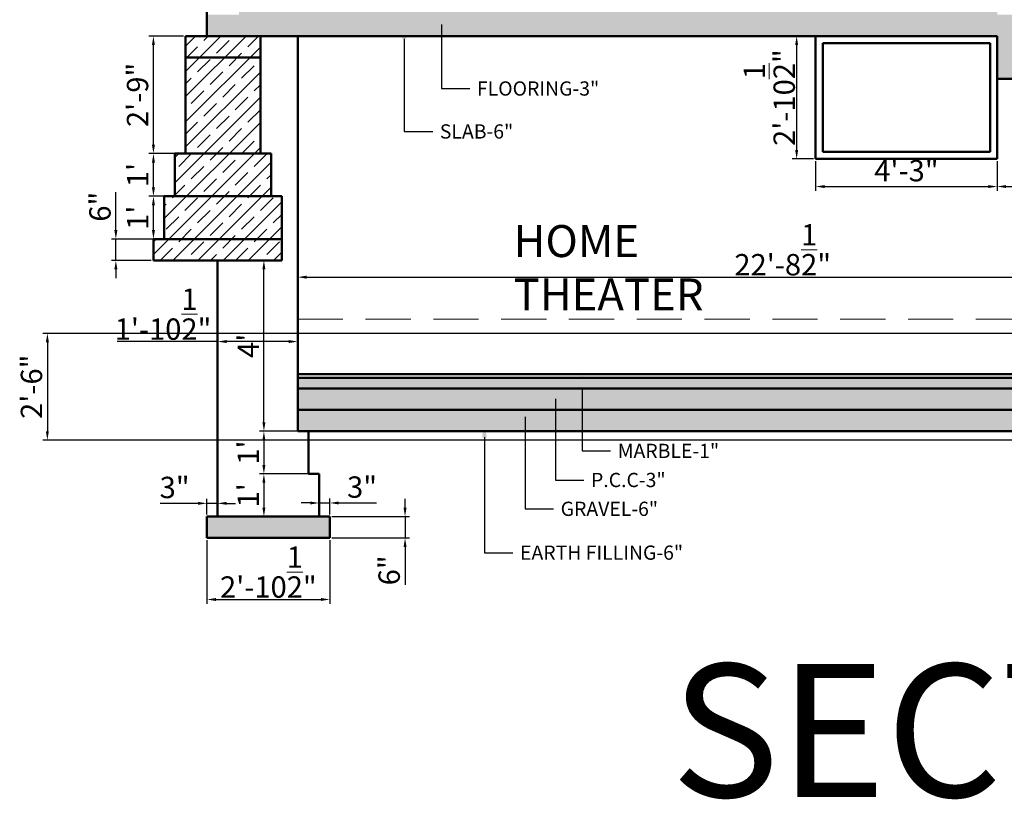
# Model space of a CAD drawing. Units: inches. Extents: x 1615 to 2231, y 1931 to 2519.
# Tile 1 of 6: x 1615 to 1892, y 1931 to 2150. Entities that reach past the tile are written whole.
import ezdxf
from ezdxf import colors
from ezdxf.entities.mleader import LeaderData, LeaderLine
from ezdxf.math import Vec2, Vec3

# ---------------------------------------------------------------- set-up
doc = ezdxf.new("R2010")
doc.units = ezdxf.units.IN
doc.linetypes.add('DASHED', pattern=[19.05, 12.7, -6.35])
for name, color, linetype, lineweight in [('A-ANNO-DIMS', 2, 'Continuous', 18), ('A-ANNO-NOTE', 3, 'Continuous', 18), ('A-ANNO-TEXT', 7, 'Continuous', 35), ('A-AREA-IDEN', 7, 'Continuous', 25), ('A-SECT', 7, 'Continuous', 50), ('A-SECT-HIDN', 8, 'DASHED', 18), ('A-WALL-PATT', 8, 'Continuous', 13), ('C-TOPO-PATT', 252, 'Continuous', 13), ('S-FNDN', 1, 'Continuous', 50), ('S-FNDN-PATT', 8, 'Continuous', 13)]:
    doc.layers.add(name, color=color, linetype=linetype, lineweight=lineweight)
doc.styles.get("Standard").update_dxf_attribs({"font": 'arial.ttf'})
doc.dimstyles.new('ISO-25', dxfattribs={"dimtxt": 6, "dimasz": 2.5, "dimexe": 1.25, "dimexo": 0.625, "dimtad": 1, "dimdec": 1, "dimlunit": 4, "dimtxsty": 'Standard', "dimcen": 2.5, "dimadec": 0, "dimazin": 0, "dimtfac": 1, "dimtdec": 1, "dimtmove": 0, "dimatfit": 3, "dimfxl": 1, "dimarcsym": 0})

# ---------------------------------------------------------------- blocks, each defined once
blk = doc.blocks.new('*D1')
at = {"layer": 'A-ANNO-DIMS', "color": 0, "lineweight": -2, "transparency": 16777216}
for p, q in [((1670.87, 2051.15), (1670.87, 2060.97)), ((1693.37, 2051.15), (1693.37, 2060.97)), ((1670.87, 2059.72), (1642.69, 2059.72)), ((1690.87, 2059.72), (1673.37, 2059.72))]:
    blk.add_line(p, q, dxfattribs=at)
at = {"layer": 'A-ANNO-DIMS', "color": 0, "lineweight": 100, "transparency": 16777216}
for points in [[(1673.37, 2060.14), (1673.37, 2059.31), (1670.87, 2059.72)], [(1690.87, 2060.14), (1690.87, 2059.31), (1693.37, 2059.72)]]:
    blk.add_solid(points, dxfattribs=at)
at = {"layer": 'Defpoints', "color": 0, "lineweight": 100, "transparency": 16777216}
for p in [(1670.87, 2059.72), (1670.87, 2050.53), (1693.37, 2050.53)]:
    blk.add_point(p, dxfattribs=at)
at = {"layer": 'A-ANNO-DIMS', "color": 0, "transparency": 16777216, "insert": (1655.53, 2067.42), "char_height": 6, "attachment_point": 5}
blk.add_mtext('1\'-10{\\H1x;\\S1/2;}"', dxfattribs=at)
blk = doc.blocks.new('*D5')
at = {"layer": 'A-ANNO-DIMS', "color": 0, "lineweight": -2, "transparency": 16777216}
for p, q in [((1642.28, 2091.03), (1642.28, 2101.71)), ((1652.24, 2088.53), (1641.03, 2088.53)), ((1642.28, 2082.53), (1642.28, 2088.53)), ((1652.24, 2082.53), (1641.03, 2082.53)), ((1642.28, 2080.03), (1642.28, 2077.53))]:
    blk.add_line(p, q, dxfattribs=at)
at = {"layer": 'A-ANNO-DIMS', "color": 0, "lineweight": 100, "transparency": 16777216}
for points in [[(1641.86, 2091.03), (1642.7, 2091.03), (1642.28, 2088.53)], [(1641.86, 2080.03), (1642.7, 2080.03), (1642.28, 2082.53)]]:
    blk.add_solid(points, dxfattribs=at)
at = {"layer": 'Defpoints', "color": 0, "lineweight": 100, "transparency": 16777216}
for p in [(1642.28, 2088.53), (1652.87, 2088.53), (1652.87, 2082.53)]:
    blk.add_point(p, dxfattribs=at)
at = {"layer": 'A-ANNO-DIMS', "color": 0, "transparency": 16777216, "insert": (1638.59, 2097.62), "char_height": 6, "attachment_point": 5, "rotation": 90}
blk.add_mtext('6"', dxfattribs=at)
blk = doc.blocks.new('*D6')
at = {"layer": 'A-ANNO-DIMS', "color": 0, "lineweight": -2, "transparency": 16777216}
for p, q in [((1655.24, 2100.53), (1651.58, 2100.53)), ((1652.83, 2091.03), (1652.83, 2098.03)), ((1655.24, 2088.53), (1651.58, 2088.53))]:
    blk.add_line(p, q, dxfattribs=at)
at = {"layer": 'A-ANNO-DIMS', "color": 0, "lineweight": 100, "transparency": 16777216}
for points in [[(1652.42, 2098.03), (1653.25, 2098.03), (1652.83, 2100.53)], [(1652.42, 2091.03), (1653.25, 2091.03), (1652.83, 2088.53)]]:
    blk.add_solid(points, dxfattribs=at)
at = {"layer": 'Defpoints', "color": 0, "lineweight": 100, "transparency": 16777216}
for p in [(1652.83, 2100.53), (1655.87, 2100.53), (1655.87, 2088.53)]:
    blk.add_point(p, dxfattribs=at)
at = {"layer": 'A-ANNO-DIMS', "color": 0, "transparency": 16777216, "insert": (1649.2, 2094.53), "char_height": 6, "attachment_point": 5, "rotation": 90}
blk.add_mtext("1'", dxfattribs=at)
blk = doc.blocks.new('*D7')
at = {"layer": 'A-ANNO-DIMS', "color": 0, "lineweight": -2, "transparency": 16777216}
for p, q in [((1658.24, 2112.53), (1651.58, 2112.53)), ((1652.83, 2103.03), (1652.83, 2110.03)), ((1658.24, 2100.53), (1651.58, 2100.53))]:
    blk.add_line(p, q, dxfattribs=at)
at = {"layer": 'A-ANNO-DIMS', "color": 0, "lineweight": 100, "transparency": 16777216}
for points in [[(1652.42, 2110.03), (1653.25, 2110.03), (1652.83, 2112.53)], [(1652.42, 2103.03), (1653.25, 2103.03), (1652.83, 2100.53)]]:
    blk.add_solid(points, dxfattribs=at)
at = {"layer": 'Defpoints', "color": 0, "lineweight": 100, "transparency": 16777216}
for p in [(1652.83, 2112.53), (1658.87, 2112.53), (1658.87, 2100.53)]:
    blk.add_point(p, dxfattribs=at)
at = {"layer": 'A-ANNO-DIMS', "color": 0, "transparency": 16777216, "insert": (1649.2, 2106.53), "char_height": 6, "attachment_point": 5, "rotation": 90}
blk.add_mtext("1'", dxfattribs=at)
blk = doc.blocks.new('*D8')
at = {"layer": 'A-ANNO-DIMS', "color": 0, "lineweight": -2, "transparency": 16777216}
for p, q in [((1661.24, 2145.53), (1651.58, 2145.53)), ((1652.83, 2115.03), (1652.83, 2143.03)), ((1661.24, 2112.53), (1651.58, 2112.53))]:
    blk.add_line(p, q, dxfattribs=at)
at = {"layer": 'A-ANNO-DIMS', "color": 0, "lineweight": 100, "transparency": 16777216}
for points in [[(1652.42, 2143.03), (1653.25, 2143.03), (1652.83, 2145.53)], [(1652.42, 2115.03), (1653.25, 2115.03), (1652.83, 2112.53)]]:
    blk.add_solid(points, dxfattribs=at)
at = {"layer": 'Defpoints', "color": 0, "lineweight": 100, "transparency": 16777216}
for p in [(1652.83, 2145.53), (1661.87, 2145.53), (1661.87, 2112.53)]:
    blk.add_point(p, dxfattribs=at)
at = {"layer": 'A-ANNO-DIMS', "color": 0, "transparency": 16777216, "insert": (1649.15, 2129.03), "char_height": 6, "attachment_point": 5, "rotation": 90}
blk.add_mtext('2\'-9"', dxfattribs=at)
blk = doc.blocks.new('*D9')
at = {"layer": 'A-ANNO-DIMS', "color": 0, "lineweight": -2, "transparency": 16777216}
for p, q in [((1693.37, 2070.69), (1693.37, 2079.07)), ((1695.87, 2077.82), (1963.37, 2077.82)), ((1965.87, 2070.69), (1965.87, 2079.07))]:
    blk.add_line(p, q, dxfattribs=at)
at = {"layer": 'A-ANNO-DIMS', "color": 0, "lineweight": 100, "transparency": 16777216}
for points in [[(1695.87, 2078.24), (1695.87, 2077.4), (1693.37, 2077.82)], [(1963.37, 2078.24), (1963.37, 2077.4), (1965.87, 2077.82)]]:
    blk.add_solid(points, dxfattribs=at)
at = {"layer": 'Defpoints', "color": 0, "lineweight": 100, "transparency": 16777216}
for p in [(1965.87, 2077.82), (1693.37, 2070.06), (1965.87, 2070.06)]:
    blk.add_point(p, dxfattribs=at)
at = {"layer": 'A-ANNO-DIMS', "color": 0, "transparency": 16777216, "insert": (1829.62, 2085.52), "char_height": 6, "attachment_point": 5}
blk.add_mtext('22\'-8{\\H1x;\\S1/2;}"', dxfattribs=at)
blk = doc.blocks.new('*D11')
at = {"layer": 'A-ANNO-DIMS', "color": 0, "lineweight": -2, "transparency": 16777216}
for p, q in [((1688.24, 2082.53), (1682.62, 2082.53)), ((1683.87, 2037.03), (1683.87, 2080.03)), ((1692.74, 2034.53), (1682.62, 2034.53))]:
    blk.add_line(p, q, dxfattribs=at)
at = {"layer": 'A-ANNO-DIMS', "color": 0, "lineweight": 100, "transparency": 16777216}
for points in [[(1683.45, 2080.03), (1684.28, 2080.03), (1683.87, 2082.53)], [(1683.45, 2037.03), (1684.28, 2037.03), (1683.87, 2034.53)]]:
    blk.add_solid(points, dxfattribs=at)
at = {"layer": 'Defpoints', "color": 0, "lineweight": 100, "transparency": 16777216}
for p in [(1683.87, 2082.53), (1688.87, 2082.53), (1693.37, 2034.53)]:
    blk.add_point(p, dxfattribs=at)
at = {"layer": 'A-ANNO-DIMS', "color": 0, "transparency": 16777216, "insert": (1680.24, 2058.53), "char_height": 6, "attachment_point": 5, "rotation": 90}
blk.add_mtext("4'", dxfattribs=at)
blk = doc.blocks.new('*D12')
at = {"layer": 'A-ANNO-DIMS', "color": 0, "lineweight": -2, "transparency": 16777216}
for p, q in [((1695.74, 2034.53), (1682.62, 2034.53)), ((1683.87, 2032.03), (1683.87, 2025.03)), ((1695.74, 2022.53), (1682.62, 2022.53))]:
    blk.add_line(p, q, dxfattribs=at)
at = {"layer": 'A-ANNO-DIMS', "color": 0, "lineweight": 100, "transparency": 16777216}
for points in [[(1683.45, 2032.03), (1684.28, 2032.03), (1683.87, 2034.53)], [(1683.45, 2025.03), (1684.28, 2025.03), (1683.87, 2022.53)]]:
    blk.add_solid(points, dxfattribs=at)
at = {"layer": 'Defpoints', "color": 0, "lineweight": 100, "transparency": 16777216}
for p in [(1696.37, 2034.53), (1683.87, 2022.53), (1696.37, 2022.53)]:
    blk.add_point(p, dxfattribs=at)
at = {"layer": 'A-ANNO-DIMS', "color": 0, "transparency": 16777216, "insert": (1680.23, 2028.53), "char_height": 6, "attachment_point": 5, "rotation": 90}
blk.add_mtext("1'", dxfattribs=at)
blk = doc.blocks.new('*D13')
at = {"layer": 'A-ANNO-DIMS', "color": 0, "lineweight": -2, "transparency": 16777216}
for p, q in [((1698.74, 2022.53), (1682.62, 2022.53)), ((1683.87, 2020.03), (1683.87, 2013.03)), ((1698.74, 2010.53), (1682.62, 2010.53))]:
    blk.add_line(p, q, dxfattribs=at)
at = {"layer": 'A-ANNO-DIMS', "color": 0, "lineweight": 100, "transparency": 16777216}
for points in [[(1683.45, 2020.03), (1684.28, 2020.03), (1683.87, 2022.53)], [(1683.45, 2013.03), (1684.28, 2013.03), (1683.87, 2010.53)]]:
    blk.add_solid(points, dxfattribs=at)
at = {"layer": 'Defpoints', "color": 0, "lineweight": 100, "transparency": 16777216}
for p in [(1699.37, 2022.53), (1683.87, 2010.53), (1699.37, 2010.53)]:
    blk.add_point(p, dxfattribs=at)
at = {"layer": 'A-ANNO-DIMS', "color": 0, "transparency": 16777216, "insert": (1680.23, 2016.53), "char_height": 6, "attachment_point": 5, "rotation": 90}
blk.add_mtext("1'", dxfattribs=at)
blk = doc.blocks.new('*D14')
at = {"layer": 'A-ANNO-DIMS', "color": 0, "lineweight": -2, "transparency": 16777216}
for p, q in [((1667.87, 2003.9), (1667.87, 1986)), ((1702.37, 2003.9), (1702.37, 1986)), ((1670.37, 1987.25), (1699.87, 1987.25))]:
    blk.add_line(p, q, dxfattribs=at)
at = {"layer": 'A-ANNO-DIMS', "color": 0, "lineweight": 100, "transparency": 16777216}
for points in [[(1670.37, 1987.67), (1670.37, 1986.84), (1667.87, 1987.25)], [(1699.87, 1987.67), (1699.87, 1986.84), (1702.37, 1987.25)]]:
    blk.add_solid(points, dxfattribs=at)
at = {"layer": 'Defpoints', "color": 0, "lineweight": 100, "transparency": 16777216}
for p in [(1667.87, 2004.53), (1702.37, 2004.53), (1702.37, 1987.25)]:
    blk.add_point(p, dxfattribs=at)
at = {"layer": 'A-ANNO-DIMS', "color": 0, "transparency": 16777216, "insert": (1685.12, 1994.95), "char_height": 6, "attachment_point": 5}
blk.add_mtext('2\'-10{\\H1x;\\S1/2;}"', dxfattribs=at)
blk = doc.blocks.new('*D15')
at = {"layer": 'A-ANNO-DIMS', "color": 0, "lineweight": -2, "transparency": 16777216}
for p, q in [((1696.87, 2014.37), (1694.37, 2014.37)), ((1699.37, 2011.15), (1699.37, 2015.62)), ((1699.37, 2014.37), (1702.37, 2014.37)), ((1702.37, 2011.15), (1702.37, 2015.62)), ((1704.87, 2014.37), (1715.51, 2014.37))]:
    blk.add_line(p, q, dxfattribs=at)
at = {"layer": 'A-ANNO-DIMS', "color": 0, "lineweight": 100, "transparency": 16777216}
for points in [[(1696.87, 2014.78), (1696.87, 2013.95), (1699.37, 2014.37)], [(1704.87, 2014.78), (1704.87, 2013.95), (1702.37, 2014.37)]]:
    blk.add_solid(points, dxfattribs=at)
at = {"layer": 'Defpoints', "color": 0, "lineweight": 100, "transparency": 16777216}
for p in [(1702.37, 2014.37), (1699.37, 2010.53), (1702.37, 2010.53)]:
    blk.add_point(p, dxfattribs=at)
at = {"layer": 'A-ANNO-DIMS', "color": 0, "transparency": 16777216, "insert": (1711.44, 2018.06), "char_height": 6, "attachment_point": 5}
blk.add_mtext('3"', dxfattribs=at)
blk = doc.blocks.new('*D16')
at = {"layer": 'A-ANNO-DIMS', "color": 0, "lineweight": -2, "transparency": 16777216}
for p, q in [((1665.37, 2014.26), (1654.72, 2014.26)), ((1667.87, 2011.15), (1667.87, 2015.51)), ((1670.87, 2014.26), (1667.87, 2014.26)), ((1670.87, 2011.15), (1670.87, 2015.51)), ((1673.37, 2014.26), (1675.87, 2014.26))]:
    blk.add_line(p, q, dxfattribs=at)
at = {"layer": 'A-ANNO-DIMS', "color": 0, "lineweight": 100, "transparency": 16777216}
for points in [[(1665.37, 2014.68), (1665.37, 2013.85), (1667.87, 2014.26)], [(1673.37, 2014.68), (1673.37, 2013.85), (1670.87, 2014.26)]]:
    blk.add_solid(points, dxfattribs=at)
at = {"layer": 'Defpoints', "color": 0, "lineweight": 100, "transparency": 16777216}
for p in [(1667.87, 2014.26), (1667.87, 2010.53), (1670.87, 2010.53)]:
    blk.add_point(p, dxfattribs=at)
at = {"layer": 'A-ANNO-DIMS', "color": 0, "transparency": 16777216, "insert": (1658.79, 2017.95), "char_height": 6, "attachment_point": 5}
blk.add_mtext('3"', dxfattribs=at)
blk = doc.blocks.new('*D23')
at = {"layer": 'A-ANNO-DIMS', "color": 0, "lineweight": -2, "transparency": 16777216}
for p, q in [((1838.24, 2145.53), (1832.28, 2145.53)), ((1833.53, 2143.03), (1833.53, 2113.53)), ((1838.24, 2111.03), (1832.28, 2111.03))]:
    blk.add_line(p, q, dxfattribs=at)
at = {"layer": 'A-ANNO-DIMS', "color": 0, "lineweight": 100, "transparency": 16777216}
for points in [[(1833.11, 2143.03), (1833.95, 2143.03), (1833.53, 2145.53)], [(1833.11, 2113.53), (1833.95, 2113.53), (1833.53, 2111.03)]]:
    blk.add_solid(points, dxfattribs=at)
at = {"layer": 'Defpoints', "color": 0, "lineweight": 100, "transparency": 16777216}
for p in [(1838.87, 2145.53), (1833.53, 2111.03), (1838.87, 2111.03)]:
    blk.add_point(p, dxfattribs=at)
at = {"layer": 'A-ANNO-DIMS', "color": 0, "transparency": 16777216, "insert": (1825.83, 2128.28), "char_height": 6, "attachment_point": 5, "rotation": 90}
blk.add_mtext('2\'-10{\\H1x;\\S1/2;}"', dxfattribs=at)
blk = doc.blocks.new('*D24')
at = {"layer": 'A-ANNO-DIMS', "color": 0, "lineweight": -2, "transparency": 16777216}
for p, q in [((1838.87, 2110.4), (1838.87, 2102.03)), ((1889.87, 2110.4), (1889.87, 2102.03)), ((1841.37, 2103.28), (1887.37, 2103.28))]:
    blk.add_line(p, q, dxfattribs=at)
at = {"layer": 'A-ANNO-DIMS', "color": 0, "lineweight": 100, "transparency": 16777216}
for points in [[(1841.37, 2103.7), (1841.37, 2102.86), (1838.87, 2103.28)], [(1887.37, 2103.7), (1887.37, 2102.86), (1889.87, 2103.28)]]:
    blk.add_solid(points, dxfattribs=at)
at = {"layer": 'Defpoints', "color": 0, "lineweight": 100, "transparency": 16777216}
for p in [(1838.87, 2111.03), (1889.87, 2111.03), (1889.87, 2103.28)]:
    blk.add_point(p, dxfattribs=at)
at = {"layer": 'A-ANNO-DIMS', "color": 0, "transparency": 16777216, "insert": (1864.37, 2106.97), "char_height": 6, "attachment_point": 5}
blk.add_mtext('4\'-3"', dxfattribs=at)
blk = doc.blocks.new('*D26')
at = {"layer": 'A-ANNO-DIMS', "color": 0, "lineweight": -2, "transparency": 16777216}
for p, q in [((1889.87, 2110.4), (1889.87, 2102.03)), ((1965.87, 2110.4), (1965.87, 2102.03)), ((1892.37, 2103.28), (1963.37, 2103.28))]:
    blk.add_line(p, q, dxfattribs=at)
at = {"layer": 'A-ANNO-DIMS', "color": 0, "lineweight": 100, "transparency": 16777216}
for points in [[(1892.37, 2103.7), (1892.37, 2102.86), (1889.87, 2103.28)], [(1963.37, 2103.7), (1963.37, 2102.86), (1965.87, 2103.28)]]:
    blk.add_solid(points, dxfattribs=at)
at = {"layer": 'Defpoints', "color": 0, "lineweight": 100, "transparency": 16777216}
for p in [(1889.87, 2111.03), (1965.87, 2111.03), (1965.87, 2103.28)]:
    blk.add_point(p, dxfattribs=at)
at = {"layer": 'A-ANNO-DIMS', "color": 0, "transparency": 16777216, "insert": (1927.87, 2106.97), "char_height": 6, "attachment_point": 5}
blk.add_mtext('6\'-4"', dxfattribs=at)
blk = doc.blocks.new('*D74')
at = {"layer": 'A-ANNO-DIMS', "color": 0, "lineweight": -2, "transparency": 16777216}
for p, q in [((1723.52, 2013.03), (1723.52, 2015.53)), ((1702.99, 2010.53), (1724.77, 2010.53)), ((1723.52, 2010.53), (1723.52, 2004.53)), ((1702.99, 2004.53), (1724.77, 2004.53)), ((1723.52, 2002.03), (1723.52, 1991.35))]:
    blk.add_line(p, q, dxfattribs=at)
at = {"layer": 'A-ANNO-DIMS', "color": 0, "lineweight": 100, "transparency": 16777216}
for points in [[(1723.1, 2013.03), (1723.94, 2013.03), (1723.52, 2010.53)], [(1723.1, 2002.03), (1723.94, 2002.03), (1723.52, 2004.53)]]:
    blk.add_solid(points, dxfattribs=at)
at = {"layer": 'Defpoints', "color": 0, "lineweight": 100, "transparency": 16777216}
for p in [(1702.37, 2010.53), (1702.37, 2004.53), (1723.52, 2004.53)]:
    blk.add_point(p, dxfattribs=at)
at = {"layer": 'A-ANNO-DIMS', "color": 0, "transparency": 16777216, "insert": (1719.83, 1995.44), "char_height": 6, "attachment_point": 5, "rotation": 90}
blk.add_mtext('6"', dxfattribs=at)
blk = doc.blocks.new('*D88')
at = {"layer": 'A-ANNO-DIMS', "color": 0, "lineweight": -2, "transparency": 16777216}
for p, q in [((2162.74, 2062.03), (1621.79, 2062.03)), ((1623.04, 2059.53), (1623.04, 2034.53)), ((2165.74, 2032.03), (1621.79, 2032.03))]:
    blk.add_line(p, q, dxfattribs=at)
at = {"layer": 'A-ANNO-DIMS', "color": 0, "lineweight": 100, "transparency": 16777216}
for points in [[(1622.62, 2059.53), (1623.46, 2059.53), (1623.04, 2062.03)], [(1622.62, 2034.53), (1623.46, 2034.53), (1623.04, 2032.03)]]:
    blk.add_solid(points, dxfattribs=at)
at = {"layer": 'Defpoints', "color": 0, "lineweight": 100, "transparency": 16777216}
for p in [(2163.37, 2062.03), (1623.04, 2032.03), (2166.37, 2032.03)]:
    blk.add_point(p, dxfattribs=at)
at = {"layer": 'A-ANNO-DIMS', "color": 0, "transparency": 16777216, "insert": (1619.35, 2047.03), "char_height": 6, "attachment_point": 5, "rotation": 90}
blk.add_mtext('2\'-6"', dxfattribs=at)

msp = doc.modelspace()

# ---------------------------------------------------------------- hatches: boundary and pattern name
at = {"layer": 'A-WALL-PATT'}
h = msp.add_hatch(dxfattribs=at)
h.set_pattern_fill('DOTS', color=256, scale=0.5)
h.paths.add_polyline_path([(2142.37, 2442.53), (1839.37, 2442.53), (1676.87, 2442.53), (1676.87, 2439.53), (2142.37, 2439.53)])
h.paths.add_polyline_path([(1889.87, 2298.53), (1676.87, 2298.53), (1676.87, 2295.53), (1889.87, 2295.53)])
h.paths.add_polyline_path([(2142.37, 2298.53), (1974.87, 2298.53), (1974.87, 2295.53), (2142.37, 2295.53)])
h.paths.add_polyline_path([(1889.87, 2154.53), (1676.87, 2154.53), (1676.87, 2151.53), (1889.87, 2151.53)])
h.paths.add_polyline_path([(1965.87, 2154.53), (1894.37, 2154.53), (1894.37, 2151.53), (1965.87, 2151.53)])
h.paths.add_polyline_path([(2142.37, 2154.53), (1974.87, 2154.53), (1974.87, 2151.53), (2142.37, 2151.53)])
h.paths.add_polyline_path([(2094.37, 2062.03), (1974.87, 2062.03), (1974.87, 2059.03), (2094.37, 2059.03)])
h.paths.add_polyline_path([(2142.37, 2062.03), (2098.87, 2062.03), (2098.87, 2059.03), (2142.37, 2059.03)])
h.paths.add_polyline_path([(1956.87, 2049.53), (1693.37, 2049.53), (1693.37, 2046.53), (1956.87, 2046.53)])
h = msp.add_hatch(dxfattribs=at)
h.set_pattern_fill('AR-CONC', color=256, scale=0.1)
h.paths.add_polyline_path([(1898.87, 2151.53), (1667.87, 2151.53), (1667.87, 2145.53), (1679.87, 2145.53), (1682.87, 2145.53), (1889.87, 2145.53), (1889.87, 2133.53), (1974.87, 2133.53), (1974.87, 2145.53), (2142.37, 2145.53), (2142.37, 2133.53), (2157.37, 2133.53), (2157.37, 2151.53), (2155.87, 2151.53), (2151.37, 2151.53), (1965.87, 2151.53), (1965.87, 2139.53), (1898.87, 2139.53)])
h.paths.add_polyline_path([(1898.87, 2295.53), (1667.87, 2295.53), (1667.87, 2277.53), (1676.87, 2277.53), (1676.87, 2289.53), (1889.87, 2289.53), (1889.87, 2277.53), (1974.87, 2277.53), (1974.87, 2289.53), (2142.37, 2289.53), (2142.37, 2277.53), (2151.37, 2277.53), (2151.37, 2295.53), (1965.87, 2295.53), (1965.87, 2283.53), (1898.87, 2283.53)])
h.paths.add_polyline_path([(2142.37, 2439.53), (1676.87, 2439.53), (1667.87, 2439.53), (1667.87, 2421.53), (1676.87, 2421.53), (1676.87, 2433.53), (1889.87, 2433.53), (1889.87, 2421.29), (1898.87, 2421.29), (1898.87, 2433.53), (1965.87, 2433.53), (1965.87, 2421.29), (1974.87, 2421.29), (1974.87, 2433.53), (2142.37, 2433.53)])
h = msp.add_hatch(dxfattribs=at)
h.set_pattern_fill('JIS_STN_1E', color=256, scale=5)
h.paths.add_polyline_path([(1688.87, 2100.53), (1655.87, 2100.53), (1655.87, 2088.53), (1688.87, 2088.53)])
h.paths.add_polyline_path([(1685.87, 2112.53), (1658.87, 2112.53), (1658.87, 2100.53), (1685.87, 2100.53)])
h.paths.add_polyline_path([(1682.87, 2139.53), (1661.87, 2139.53), (1661.87, 2112.53), (1682.87, 2112.53)])
h.paths.add_polyline_path([(1688.87, 2088.53), (1655.87, 2088.53), (1652.87, 2088.53), (1652.87, 2082.53), (1688.87, 2082.53)])
h.paths.add_polyline_path([(1682.87, 2145.53), (1679.87, 2145.53), (1676.87, 2145.53), (1661.87, 2145.53), (1661.87, 2139.53), (1682.87, 2139.53)])
h.paths.add_polyline_path([(1974.87, 2057.03), (1956.87, 2057.03), (1956.87, 2044.03), (1974.87, 2044.03)])
h.paths.add_polyline_path([(1974.87, 2060.03), (1956.87, 2060.03), (1956.87, 2057.03), (1974.87, 2057.03)])
h.paths.add_polyline_path([(1980.87, 2032.03), (1950.87, 2032.03), (1950.87, 2020.03), (1980.87, 2020.03)])
h.paths.add_polyline_path([(1977.87, 2044.03), (1953.87, 2044.03), (1953.87, 2032.03), (1977.87, 2032.03)])
h.paths.add_polyline_path([(1983.87, 2020.03), (1947.87, 2020.03), (1947.87, 2008.03), (1983.87, 2008.03)])
h.paths.add_polyline_path([(2104.12, 2056.03), (2089.12, 2056.03), (2089.12, 2032.03), (2104.12, 2032.03)])
h.paths.add_polyline_path([(2104.12, 2059.03), (2089.12, 2059.03), (2089.12, 2056.03), (2104.12, 2056.03)])
h.paths.add_polyline_path([(2105.62, 2032.03), (2087.62, 2032.03), (2087.62, 2020.03), (2105.62, 2020.03)])
h.paths.add_polyline_path([(2107.12, 2020.03), (2086.12, 2020.03), (2086.12, 2008.03), (2107.12, 2008.03)])
h.paths.add_polyline_path([(2169.37, 2032.03), (2139.37, 2032.03), (2139.37, 2020.03), (2169.37, 2020.03)])
h.paths.add_polyline_path([(2172.37, 2020.03), (2136.37, 2020.03), (2136.37, 2008.03), (2172.37, 2008.03)])
h.paths.add_polyline_path([(2166.37, 2062.03), (2163.37, 2062.03), (2163.37, 2089.03), (2160.37, 2089.03), (2160.37, 2112.53), (2157.37, 2112.53), (2157.37, 2133.53), (2142.37, 2133.53), (2142.37, 2032.03), (2166.37, 2032.03)])
at = {"layer": 'C-TOPO-PATT'}
h = msp.add_hatch(dxfattribs=at)
h.set_pattern_fill('GRAVEL', color=256, scale=0.5, angle=27)
h.paths.add_polyline_path([(1956.87, 2046.53), (1693.37, 2046.53), (1693.37, 2040.53), (1953.87, 2040.53), (1953.87, 2044.03), (1956.87, 2044.03)])
h.paths.add_polyline_path([(2089.12, 2059.03), (1974.87, 2059.03), (1974.87, 2053.03), (2089.12, 2053.03)])
h.paths.add_polyline_path([(2142.37, 2059.03), (2104.12, 2059.03), (2104.12, 2053.03), (2142.37, 2053.03)])
h.paths.add_polyline_path([(2195.62, 2124.53), (2157.37, 2124.53), (2157.37, 2118.53), (2195.62, 2118.53)])
h = msp.add_hatch(dxfattribs=at)
h.set_pattern_fill('EARTH', color=256, angle=27)
h.paths.add_polyline_path([(1953.87, 2040.53), (1693.37, 2040.53), (1693.37, 2034.53), (1696.37, 2034.53), (1953.87, 2034.53)])
h.paths.add_polyline_path([(2089.12, 2053.03), (1974.87, 2053.03), (1974.87, 2047.03), (2089.12, 2047.03)])
h.paths.add_polyline_path([(2142.37, 2053.03), (2104.12, 2053.03), (2104.12, 2047.03), (2142.37, 2047.03)])
at = {"layer": 'S-FNDN-PATT'}
h = msp.add_hatch(dxfattribs=at)
h.set_pattern_fill('AR-CONC', color=256, scale=0.1)
h.paths.add_polyline_path([(1702.37, 2010.53), (1667.87, 2010.53), (1667.87, 2004.53), (1702.37, 2004.53)])
h.paths.add_polyline_path([(1986.87, 2008.03), (1944.87, 2008.03), (1944.87, 2002.03), (1986.87, 2002.03)])
h.paths.add_polyline_path([(2108.62, 2008.03), (2084.62, 2008.03), (2084.62, 2002.03), (2108.62, 2002.03)])
h.paths.add_polyline_path([(2175.37, 2008.03), (2133.37, 2008.03), (2133.37, 2002.03), (2175.37, 2002.03)])

# ---------------------------------------------------------------- linework, layer by layer
at = {"layer": 'A-SECT'}
for p, q in [((1667.87, 2476.53), (1667.87, 2145.53)), ((1679.87, 2145.53), (1661.87, 2145.53)), ((1661.87, 2145.53), (1661.87, 2112.53)), ((1667.87, 2145.53), (1676.87, 2145.53)), ((1676.87, 2145.53), (1889.87, 2145.53)), ((1682.87, 2145.53), (1679.87, 2145.53)), ((1682.87, 2139.53), (1682.87, 2145.53)), ((1693.37, 2145.53), (1693.37, 2034.53)), ((1838.87, 2145.53), (1838.87, 2111.03)), ((1889.87, 2145.53), (1889.87, 2133.53)), ((1840.87, 2143.53), (1887.87, 2143.53)), ((1840.87, 2143.53), (1840.87, 2113.03)), ((1887.87, 2143.53), (1887.87, 2133.53)), ((1682.87, 2139.53), (1661.87, 2139.53)), ((1682.87, 2139.53), (1682.87, 2112.53)), ((1887.87, 2113.03), (1887.87, 2133.53)), ((1889.87, 2133.53), (1974.87, 2133.53)), ((1889.87, 2111.03), (1889.87, 2133.53)), ((1838.87, 2111.03), (1889.87, 2111.03)), ((1840.87, 2113.03), (1887.87, 2113.03)), ((1693.37, 2050.53), (1956.87, 2050.53)), ((1693.37, 2049.53), (1956.87, 2049.53)), ((1693.37, 2046.53), (1956.87, 2046.53)), ((1693.37, 2040.53), (1953.87, 2040.53))]:
    msp.add_line(p, q, dxfattribs=at)
at = {"layer": 'A-SECT-HIDN'}
msp.add_line((1693.37, 2066.03), (1965.87, 2066.03), dxfattribs=at)
at = {"layer": 'S-FNDN'}
for p, q in [((1685.87, 2112.53), (1658.87, 2112.53)), ((1658.87, 2112.53), (1658.87, 2100.53)), ((1685.87, 2112.53), (1685.87, 2100.53)), ((1688.87, 2100.53), (1655.87, 2100.53)), ((1655.87, 2100.53), (1655.87, 2088.53)), ((1688.87, 2100.53), (1688.87, 2088.53)), ((1688.87, 2088.53), (1652.87, 2088.53)), ((1652.87, 2088.53), (1652.87, 2082.53)), ((1688.87, 2082.53), (1688.87, 2088.53)), ((1652.87, 2082.53), (1688.87, 2082.53)), ((1670.87, 2082.53), (1670.87, 2010.53)), ((1696.37, 2034.53), (1693.37, 2034.53)), ((1696.37, 2034.53), (1696.37, 2022.53)), ((1696.37, 2034.53), (1953.87, 2034.53)), ((1699.37, 2022.53), (1696.37, 2022.53)), ((1699.37, 2022.53), (1699.37, 2010.53)), ((1702.37, 2010.53), (1667.87, 2010.53)), ((1667.87, 2010.53), (1667.87, 2004.53)), ((1702.37, 2004.53), (1702.37, 2010.53)), ((1667.87, 2004.53), (1702.37, 2004.53))]:
    msp.add_line(p, q, dxfattribs=at)

# ---------------------------------------------------------------- texts
at = {"layer": 'A-ANNO-TEXT'}
msp.add_text('SECTION', height=37.358, dxfattribs=at).set_placement((1798.24, 1931.77))
at = {"layer": 'A-AREA-IDEN', "insert": (1754.02, 2092.46), "char_height": 9, "attachment_point": 1}
msp.add_mtext_dynamic_manual_height_columns('HOME THEATER', width=38.6979, gutter_width=12.5, heights=[0], dxfattribs=at)

# ---------------------------------------------------------------- dimensions: what is measured, and where the dimension line sits
at = {"layer": 'A-ANNO-DIMS'}
for base, p1, p2, override, picture, middle in [((1652.83, 2145.53), (1661.87, 2112.53), (1661.87, 2145.53), {"dimclrd": 0, "dimclre": 0, "dimclrt": 0}, '*D8', (1649.15, 2129.03)), ((1833.53, 2111.03), (1838.87, 2145.53), (1838.87, 2111.03), {"dimclrd": 0, "dimclre": 0, "dimclrt": 0}, '*D23', (1825.83, 2128.28)), ((1652.83, 2112.53), (1658.87, 2100.53), (1658.87, 2112.53), {"dimclrd": 0, "dimclre": 0, "dimclrt": 0}, '*D7', (1649.2, 2106.53)), ((1642.28, 2088.53), (1652.87, 2082.53), (1652.87, 2088.53), {"dimclrd": 0, "dimclre": 0, "dimclrt": 0}, '*D5', (1638.59, 2097.62)), ((1652.83, 2100.53), (1655.87, 2088.53), (1655.87, 2100.53), {"dimclrd": 0, "dimclre": 0, "dimclrt": 0}, '*D6', (1649.2, 2094.53)), ((1683.87, 2082.53), (1693.37, 2034.53), (1688.87, 2082.53), {"dimclrd": 0, "dimclre": 0, "dimclrt": 0}, '*D11', (1680.24, 2058.53)), ((1623.04, 2032.03), (2163.37, 2062.03), (2166.37, 2032.03), {"dimdec": 1, "dimlfac": 1, "dimrnd": 0, "dimzin": 1, "dimdsep": 46, "dimlunit": 4, "dimfrac": 2}, '*D88', (1619.35, 2047.03)), ((1683.87, 2022.53), (1696.37, 2034.53), (1696.37, 2022.53), {"dimclrd": 0, "dimclre": 0, "dimclrt": 0}, '*D12', (1680.23, 2028.53)), ((1683.87, 2010.53), (1699.37, 2022.53), (1699.37, 2010.53), {"dimclrd": 0, "dimclre": 0, "dimclrt": 0}, '*D13', (1680.23, 2016.53)), ((1723.52, 2004.53), (1702.37, 2010.53), (1702.37, 2004.53), {"dimclrd": 0, "dimclre": 0, "dimclrt": 0}, '*D74', (1719.83, 1995.44))]:
    dim = msp.add_linear_dim(base=base, p1=p1, p2=p2, angle=90, dimstyle='ISO-25', override=override, dxfattribs=at)
    dim.commit()
    dim.dimension.update_dxf_attribs({"geometry": picture, "text_midpoint": middle})
for base, p1, p2, picture, middle in [((1889.87, 2103.28), (1838.87, 2111.03), (1889.87, 2111.03), '*D24', (1864.37, 2106.97)), ((1965.87, 2103.28), (1889.87, 2111.03), (1965.87, 2111.03), '*D26', (1927.87, 2106.97)), ((1965.87, 2077.82), (1693.37, 2070.06), (1965.87, 2070.06), '*D9', (1829.62, 2085.52)), ((1670.87, 2059.72), (1693.37, 2050.53), (1670.87, 2050.53), '*D1', (1655.53, 2067.42)), ((1667.87, 2014.26), (1670.87, 2010.53), (1667.87, 2010.53), '*D16', (1658.79, 2017.95)), ((1702.37, 2014.37), (1699.37, 2010.53), (1702.37, 2010.53), '*D15', (1711.44, 2018.06)), ((1702.37, 1987.25), (1667.87, 2004.53), (1702.37, 2004.53), '*D14', (1685.12, 1994.95))]:
    dim = msp.add_linear_dim(base=base, p1=p1, p2=p2, dimstyle='ISO-25', override={"dimclrd": 0, "dimclre": 0, "dimclrt": 0}, dxfattribs=at)
    dim.commit()
    dim.dimension.update_dxf_attribs({"geometry": picture, "text_midpoint": middle})

# ---------------------------------------------------------------- leaders
at = {"layer": 'A-ANNO-NOTE'}
ml = msp.add_multileader_mtext('Standard', dxfattribs=at)
ml.set_content('FLOORING-3"', color=256)
ml.set_leader_properties()
ml.build(insert=Vec2(0, 0))
ctx = ml.context
ctx.base_point, ctx.plane_origin = Vec3(1741.72, 2130.79), Vec3(1733.72, 2152.85)
notes = []
notes.append((ctx, [(0, (1, 1, 0), (1733.72, 2130.79), (1, 0), 8, [(0, [(1733.72, 2152.85)], 0, [])])]))
ctx.mtext.insert, ctx.mtext.flow_direction = Vec3(1743.72, 2132.83), 5
ml = msp.add_multileader_mtext('Standard', dxfattribs=at)
ml.set_content('SLAB-6"', color=256)
ml.set_leader_properties()
ml.build(insert=Vec2(0, 0))
ctx = ml.context
ctx.base_point, ctx.plane_origin = Vec3(1731.29, 2118.73), Vec3(1723.29, 2148.8)
notes.append((ctx, [(0, (1, 1, 0), (1723.29, 2118.73), (1, 0), 8, [(0, [(1723.29, 2148.8)], 0, [])])]))
ctx.mtext.insert, ctx.mtext.flow_direction = Vec3(1733.29, 2120.76), 5
ml = msp.add_multileader_mtext('Standard', dxfattribs=at)
ml.set_content('MARBLE-1"', color=256)
ml.set_leader_properties()
ml.build(insert=Vec2(0, 0))
ctx = ml.context
ctx.base_point, ctx.plane_origin = Vec3(1781.27, 2029), Vec3(1773.27, 2050.53)
notes.append((ctx, [(0, (1, 1, 0), (1773.27, 2029), (1, 0), 8, [(0, [(1773.27, 2050.53)], 0, [])])]))
ctx.mtext.insert, ctx.mtext.flow_direction = Vec3(1783.27, 2031), 5
ml = msp.add_multileader_mtext('Standard', dxfattribs=at)
ml.set_content('P.C.C-3"', color=256)
ml.set_leader_properties()
ml.build(insert=Vec2(0, 0))
ctx = ml.context
ctx.base_point, ctx.plane_origin = Vec3(1773.76, 2020.8), Vec3(1765.76, 2047.59)
notes.append((ctx, [(0, (1, 1, 0), (1765.76, 2020.8), (1, 0), 8, [(0, [(1765.76, 2047.59)], 0, [])])]))
ctx.mtext.insert, ctx.mtext.flow_direction = Vec3(1775.76, 2022.83), 5
ml = msp.add_multileader_mtext('Standard', dxfattribs=at)
ml.set_content('GRAVEL-6"', color=256)
ml.set_leader_properties()
ml.build(insert=Vec2(0, 0))
ctx = ml.context
ctx.base_point, ctx.plane_origin = Vec3(1765.23, 2012.69), Vec3(1757.23, 2042.56)
notes.append((ctx, [(0, (1, 1, 0), (1757.23, 2012.69), (1, 0), 8, [(0, [(1757.23, 2042.56)], 0, [])])]))
ctx.mtext.insert, ctx.mtext.flow_direction = Vec3(1767.23, 2014.73), 5
ml = msp.add_multileader_mtext('Standard', dxfattribs=at)
ml.set_content('EARTH FILLING-6"', color=256)
ml.set_leader_properties()
ml.build(insert=Vec2(0, 0))
ctx = ml.context
ctx.base_point, ctx.plane_origin = Vec3(1753.82, 2000.38), Vec3(1745.82, 2036.86)
notes.append((ctx, [(0, (1, 1, 0), (1745.82, 2000.38), (1, 0), 8, [(0, [(1745.82, 2036.86)], 0, [])])]))
ctx.mtext.insert, ctx.mtext.flow_direction = Vec3(1755.82, 2002.42), 5
for ctx, leaders in notes:
    for number, flags, end, landing, length, lines in leaders:
        leader = LeaderData()
        leader.index, (leader.has_last_leader_line, leader.has_dogleg_vector, leader.attachment_direction) = number, flags
        leader.last_leader_point, leader.dogleg_vector, leader.dogleg_length = Vec3(end), Vec3(landing), length
        for number, points, colour, breaks in lines:
            line = LeaderLine()
            line.index, line.vertices, line.color, line.breaks = number, Vec3.list(points), colors.encode_raw_color(colour), breaks
            leader.lines.append(line)
        ctx.leaders.append(leader)

doc.saveas('drawing.dxf')
